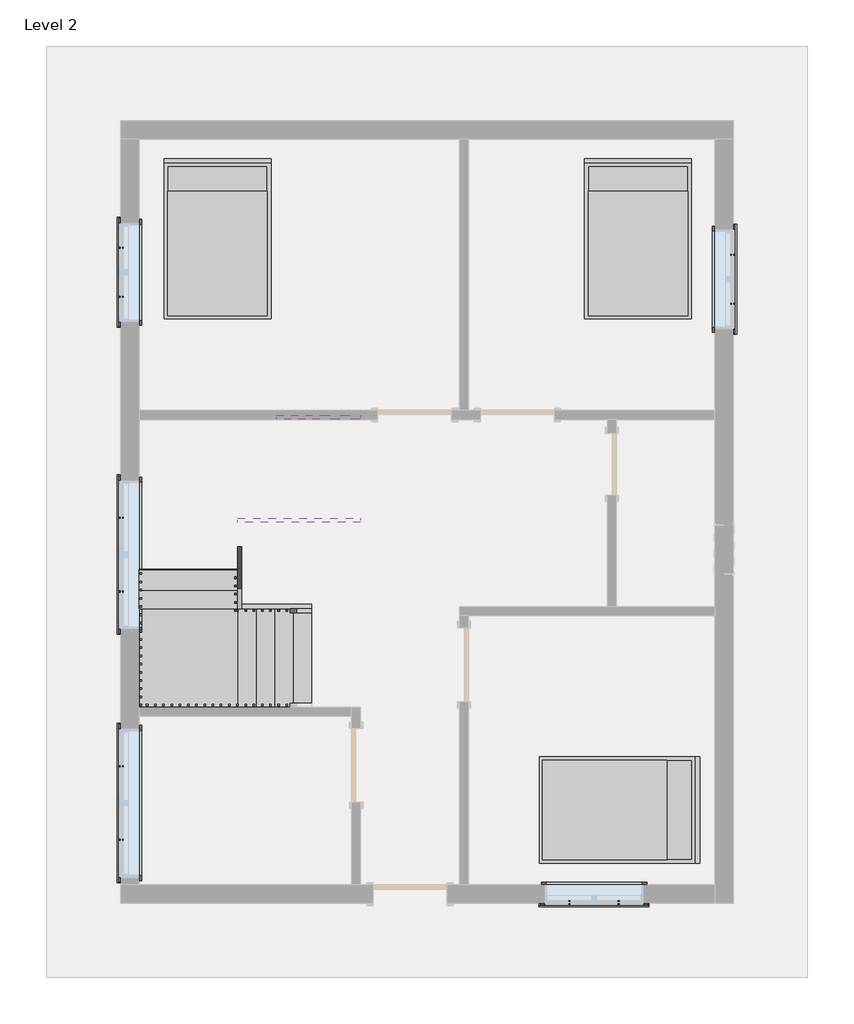
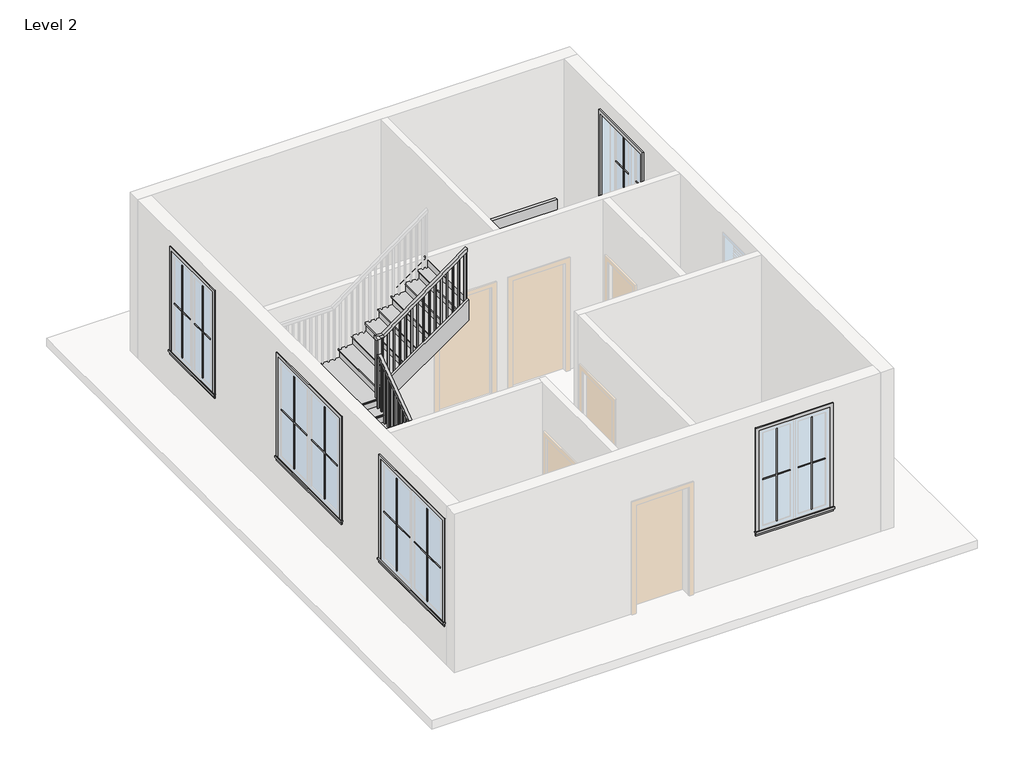
# One storey, part 3 of 3: 20 proxies, 5 members, 3 furniture elements, 1 railing, 1 stair flight.
"""IFC4 building model written with IfcOpenShell, lengths in millimetres."""

from ifc_helpers import new_model, si_unit, frame, origin, place, context, project, spatial, polyline, outline, extrude, faceted_brep, transform, mapped, element, save
from components import muntin_pattern_2x2_muntin_pattern_2x2_0a037076, muntin_pattern_2x2_muntin_pattern_2x2_e6f69628, muntin_pattern_2x2_muntin_pattern_2x2_2b4d9f72, muntin_pattern_2x2_muntin_pattern_2x2_ef995ed3, trim_window_exterior_flat_with_sill_b601e94a, trim_window_exterior_flat_with_sill_b7e4d11c, trim_window_interior_flat_picture_frame_bfefb25c, trim_window_interior_flat_picture_frame_936b8d2a, bed_17739_bed_17739_15c61121, stair_flight_7559bbc3

model = new_model("IFC4")

# Units and contexts
model_context = context("Model", 3, world=origin())
ifc_project = project(units=[si_unit("LENGTHUNIT", "METRE", prefix="MILLI")], contexts=[model_context])

# Site, building, storey
site = spatial("IfcSite", under=ifc_project)
building = spatial("IfcBuilding", under=site)
storey = spatial("IfcBuildingStorey", under=building, Name="Level 2", Elevation=3048.0)

# Proxies
placement = place(None, origin())
muntin_pattern_2x2_muntin_pattern_2x2_shape = muntin_pattern_2x2_muntin_pattern_2x2_0a037076(model_context)
element("IfcBuildingElementProxy", 1, Name="Muntin Pattern_2x2 : Muntin Pattern_2x2", ObjectType="Muntin Pattern_2x2 : Muntin Pattern_2x2", at=placement, inside=storey, context=model_context, shape_type="MappedRepresentation", body=[
    mapped(muntin_pattern_2x2_muntin_pattern_2x2_shape, transform((-5035.7855391, -4380.9248761, 4032.25), x_axis=(0.0, 1.0, 0.0), y_axis=(-1.0, 0.0, 0.0), z_axis=(0.0, 0.0, 1.0))),
])
element("IfcBuildingElementProxy", 2, Name="Muntin Pattern_2x2 : Muntin Pattern_2x2", ObjectType="Muntin Pattern_2x2 : Muntin Pattern_2x2", at=placement, inside=storey, context=model_context, shape_type="MappedRepresentation", body=[
    mapped(muntin_pattern_2x2_muntin_pattern_2x2_shape, transform((-5035.7855391, -1310.6998761, 4032.25), x_axis=(0.0, 1.0, 0.0), y_axis=(-1.0, 0.0, 0.0), z_axis=(0.0, 0.0, 1.0))),
])
muntin_pattern_2x2_muntin_pattern_2x2_2_shape = muntin_pattern_2x2_muntin_pattern_2x2_e6f69628(model_context)
element("IfcBuildingElementProxy", 3, Name="Muntin Pattern_2x2 : Muntin Pattern_2x2", ObjectType="Muntin Pattern_2x2 : Muntin Pattern_2x2", at=placement, inside=storey, context=model_context, shape_type="MappedRepresentation", body=[
    mapped(muntin_pattern_2x2_muntin_pattern_2x2_2_shape, transform((-5035.7855391, -3469.6998761, 4032.25), x_axis=(0.0, -1.0, 0.0), y_axis=(1.0, 0.0, 0.0), z_axis=(0.0, 0.0, 1.0))),
])
element("IfcBuildingElementProxy", 4, Name="Muntin Pattern_2x2 : Muntin Pattern_2x2", ObjectType="Muntin Pattern_2x2 : Muntin Pattern_2x2", at=placement, inside=storey, context=model_context, shape_type="MappedRepresentation", body=[
    mapped(muntin_pattern_2x2_muntin_pattern_2x2_2_shape, transform((-5035.7855391, -399.4748761, 4032.25), x_axis=(0.0, -1.0, 0.0), y_axis=(1.0, 0.0, 0.0), z_axis=(0.0, 0.0, 1.0))),
])
muntin_pattern_2x2_muntin_pattern_2x2_3_shape = muntin_pattern_2x2_muntin_pattern_2x2_2b4d9f72(model_context)
element("IfcBuildingElementProxy", 5, Name="Muntin Pattern_2x2 : Muntin Pattern_2x2", ObjectType="Muntin Pattern_2x2 : Muntin Pattern_2x2", at=placement, inside=storey, context=model_context, shape_type="MappedRepresentation", body=[
    mapped(muntin_pattern_2x2_muntin_pattern_2x2_3_shape, transform((1115.7769609, -5157.2123761, 4032.25), x_axis=(-1.0, 0.0, 0.0), y_axis=(0.0, -1.0, 0.0), z_axis=(0.0, 0.0, 1.0))),
])
element("IfcBuildingElementProxy", 6, Name="Muntin Pattern_2x2 : Muntin Pattern_2x2", ObjectType="Muntin Pattern_2x2 : Muntin Pattern_2x2", at=placement, inside=storey, context=model_context, shape_type="MappedRepresentation", body=[
    mapped(muntin_pattern_2x2_muntin_pattern_2x2_3_shape, transform((2527.0644609, 2851.7251239, 4032.25), x_axis=(0.0, -1.0, 0.0), y_axis=(1.0, 0.0, 0.0), z_axis=(0.0, 0.0, 1.0))),
])
element("IfcBuildingElementProxy", 7, Name="Muntin Pattern_2x2 : Muntin Pattern_2x2", ObjectType="Muntin Pattern_2x2 : Muntin Pattern_2x2", at=placement, inside=storey, context=model_context, shape_type="MappedRepresentation", body=[
    mapped(muntin_pattern_2x2_muntin_pattern_2x2_3_shape, transform((-5035.7855391, 2331.0251239, 4032.25), x_axis=(0.0, 1.0, 0.0), y_axis=(-1.0, 0.0, 0.0), z_axis=(0.0, 0.0, 1.0))),
])
muntin_pattern_2x2_muntin_pattern_2x2_4_shape = muntin_pattern_2x2_muntin_pattern_2x2_ef995ed3(model_context)
element("IfcBuildingElementProxy", 8, Name="Muntin Pattern_2x2 : Muntin Pattern_2x2", ObjectType="Muntin Pattern_2x2 : Muntin Pattern_2x2", at=placement, inside=storey, context=model_context, shape_type="MappedRepresentation", body=[
    mapped(muntin_pattern_2x2_muntin_pattern_2x2_4_shape, transform((509.3519609, -5157.2123761, 4032.25), x_axis=(1.0, 0.0, 0.0), y_axis=(0.0, 1.0, 0.0), z_axis=(0.0, 0.0, 1.0))),
])
element("IfcBuildingElementProxy", 9, Name="Muntin Pattern_2x2 : Muntin Pattern_2x2", ObjectType="Muntin Pattern_2x2 : Muntin Pattern_2x2", at=placement, inside=storey, context=model_context, shape_type="MappedRepresentation", body=[
    mapped(muntin_pattern_2x2_muntin_pattern_2x2_4_shape, transform((2527.0644609, 2245.3001239, 4032.25), x_axis=(0.0, 1.0, 0.0), y_axis=(-1.0, 0.0, 0.0), z_axis=(0.0, 0.0, 1.0))),
])
element("IfcBuildingElementProxy", 10, Name="Muntin Pattern_2x2 : Muntin Pattern_2x2", ObjectType="Muntin Pattern_2x2 : Muntin Pattern_2x2", at=placement, inside=storey, context=model_context, shape_type="MappedRepresentation", body=[
    mapped(muntin_pattern_2x2_muntin_pattern_2x2_4_shape, transform((-5035.7855391, 2937.4501239, 4032.25), x_axis=(0.0, -1.0, 0.0), y_axis=(1.0, 0.0, 0.0), z_axis=(0.0, 0.0, 1.0))),
])
trim_window_exterior_flat_with_sill_shape = trim_window_exterior_flat_with_sill_b601e94a(model_context)
element("IfcBuildingElementProxy", 11, Name="Trim-Window-Exterior-Flat : with Sill", ObjectType="Trim-Window-Exterior-Flat : with Sill", at=placement, inside=storey, context=model_context, shape_type="MappedRepresentation", body=[
    mapped(trim_window_exterior_flat_with_sill_shape, transform((-5045.3105391, -3925.3123761, 5791.2), x_axis=(0.0, -1.0, 0.0), y_axis=(0.0, 0.0, 1.0), z_axis=(-1.0, 0.0, 0.0))),
])
element("IfcBuildingElementProxy", 12, Name="Trim-Window-Exterior-Flat : with Sill", ObjectType="Trim-Window-Exterior-Flat : with Sill", at=placement, inside=storey, context=model_context, shape_type="MappedRepresentation", body=[
    mapped(trim_window_exterior_flat_with_sill_shape, transform((-5045.3105391, -855.0873761, 5791.2), x_axis=(0.0, -1.0, 0.0), y_axis=(0.0, 0.0, 1.0), z_axis=(-1.0, 0.0, 0.0))),
])
trim_window_exterior_flat_with_sill_2_shape = trim_window_exterior_flat_with_sill_b7e4d11c(model_context)
element("IfcBuildingElementProxy", 13, Name="Trim-Window-Exterior-Flat : with Sill", ObjectType="Trim-Window-Exterior-Flat : with Sill", at=placement, inside=storey, context=model_context, shape_type="MappedRepresentation", body=[
    mapped(trim_window_exterior_flat_with_sill_2_shape, transform((812.5644609, -5166.7373761, 5791.2), x_axis=(1.0, 0.0, 0.0), y_axis=(0.0, 0.0, 1.0), z_axis=(0.0, -1.0, 0.0))),
])
element("IfcBuildingElementProxy", 14, Name="Trim-Window-Exterior-Flat : with Sill", ObjectType="Trim-Window-Exterior-Flat : with Sill", at=placement, inside=storey, context=model_context, shape_type="MappedRepresentation", body=[
    mapped(trim_window_exterior_flat_with_sill_2_shape, transform((2536.5894609, 2548.5126239, 5791.2), x_axis=(0.0, 1.0, 0.0), y_axis=(0.0, 0.0, 1.0), z_axis=(1.0, 0.0, 0.0))),
])
element("IfcBuildingElementProxy", 15, Name="Trim-Window-Exterior-Flat : with Sill", ObjectType="Trim-Window-Exterior-Flat : with Sill", at=placement, inside=storey, context=model_context, shape_type="MappedRepresentation", body=[
    mapped(trim_window_exterior_flat_with_sill_2_shape, transform((-5045.3105391, 2634.2376239, 5791.2), x_axis=(0.0, -1.0, 0.0), y_axis=(0.0, 0.0, 1.0), z_axis=(-1.0, 0.0, 0.0))),
])
trim_window_interior_flat_picture_frame_shape = trim_window_interior_flat_picture_frame_bfefb25c(model_context)
element("IfcBuildingElementProxy", 16, Name="Trim-Window-Interior-Flat : Picture Frame", ObjectType="Trim-Window-Interior-Flat : Picture Frame", at=placement, inside=storey, context=model_context, shape_type="MappedRepresentation", body=[
    mapped(trim_window_interior_flat_picture_frame_shape, transform((-4816.7105391, -3925.3123761, 5791.2), x_axis=(0.0, 1.0, 0.0), y_axis=(0.0, 0.0, 1.0), z_axis=(1.0, 0.0, 0.0))),
])
element("IfcBuildingElementProxy", 17, Name="Trim-Window-Interior-Flat : Picture Frame", ObjectType="Trim-Window-Interior-Flat : Picture Frame", at=placement, inside=storey, context=model_context, shape_type="MappedRepresentation", body=[
    mapped(trim_window_interior_flat_picture_frame_shape, transform((-4816.7105391, -855.0873761, 5791.2), x_axis=(0.0, 1.0, 0.0), y_axis=(0.0, 0.0, 1.0), z_axis=(1.0, 0.0, 0.0))),
])
trim_window_interior_flat_picture_frame_2_shape = trim_window_interior_flat_picture_frame_936b8d2a(model_context)
element("IfcBuildingElementProxy", 18, Name="Trim-Window-Interior-Flat : Picture Frame", ObjectType="Trim-Window-Interior-Flat : Picture Frame", at=placement, inside=storey, context=model_context, shape_type="MappedRepresentation", body=[
    mapped(trim_window_interior_flat_picture_frame_2_shape, transform((812.5644609, -4938.1373761, 5791.2), x_axis=(-1.0, 0.0, 0.0), y_axis=(0.0, 0.0, 1.0), z_axis=(0.0, 1.0, 0.0))),
])
element("IfcBuildingElementProxy", 19, Name="Trim-Window-Interior-Flat : Picture Frame", ObjectType="Trim-Window-Interior-Flat : Picture Frame", at=placement, inside=storey, context=model_context, shape_type="MappedRepresentation", body=[
    mapped(trim_window_interior_flat_picture_frame_2_shape, transform((2307.9894609, 2548.5126239, 5791.2), x_axis=(0.0, -1.0, 0.0), y_axis=(0.0, 0.0, 1.0), z_axis=(-1.0, 0.0, 0.0))),
])
element("IfcBuildingElementProxy", 20, Name="Trim-Window-Interior-Flat : Picture Frame", ObjectType="Trim-Window-Interior-Flat : Picture Frame", at=placement, inside=storey, context=model_context, shape_type="MappedRepresentation", body=[
    mapped(trim_window_interior_flat_picture_frame_2_shape, transform((-4816.7105391, 2634.2376239, 5791.2), x_axis=(0.0, 1.0, 0.0), y_axis=(0.0, 0.0, 1.0), z_axis=(1.0, 0.0, 0.0))),
])

# Furniture
bed_17739_bed_17739_shape = bed_17739_bed_17739_15c61121(model_context)
element("IfcFurniture", 21, ObjectType="Bed_17739 : Bed_17739", at=placement, inside=storey, context=model_context, shape_type="MappedRepresentation", body=[
    mapped(bed_17739_bed_17739_shape, transform((-3845.1605391, 3024.7626239, 3048.0), x_axis=(1.0, 0.0, 0.0), y_axis=(0.0, 1.0, 0.0), z_axis=(0.0, 0.0, 1.0))),
])
element("IfcFurniture", 22, ObjectType="Bed_17739 : Bed_17739", at=placement, inside=storey, context=model_context, shape_type="MappedRepresentation", body=[
    mapped(bed_17739_bed_17739_shape, transform((1355.4894609, 3024.7626239, 3048.0), x_axis=(1.0, 0.0, 0.0), y_axis=(0.0, 1.0, 0.0), z_axis=(0.0, 0.0, 1.0))),
])
element("IfcFurniture", 23, ObjectType="Bed_17739 : Bed_17739", at=placement, inside=storey, context=model_context, shape_type="MappedRepresentation", body=[
    mapped(bed_17739_bed_17739_shape, transform((1101.4894609, -4011.0373761, 3048.0), x_axis=(0.0, -1.0, 0.0), y_axis=(1.0, 0.0, 0.0), z_axis=(0.0, 0.0, 1.0))),
])

# Members
element("IfcMember", 24, ObjectType="Stringer - 2\" Width", at=placement, inside=storey, context=model_context, shape_type="SweptSolid", body=[
    extrude(outline(polyline([(3048.0, -2683.1105391), (3198.5087903, -2683.1105391), (3198.5087903, -3112.2707489), (3048.0, -2897.7957228), (3048.0, -2683.1105391)])), frame((0.0, -2791.8373761, 0.0), z_axis=(0.0, 1.0, 0.0), x_axis=(0.0, 0.0, 1.0)), (0.0, 0.0, 1.0), 50.8),
])
element("IfcMember", 25, ObjectType="Stringer - 2\" Width", at=placement, inside=storey, context=model_context, shape_type="SweptSolid", body=[
    extrude(outline(polyline([(5375.4856495, -2580.7583047), (5731.4489938, -2073.5105391), (6103.8117181, -2073.5105391), (5375.4856495, -3111.3751869), (5375.4856495, -2580.7583047)])), frame((0.0, 814.9626239, 0.0), z_axis=(0.0, 1.0, 0.0), x_axis=(0.0, 0.0, 1.0)), (0.0, 0.0, 1.0), 50.8),
])
element("IfcMember", 26, ObjectType="Stringer - 2\" Width", at=placement, inside=storey, context=model_context, shape_type="SweptSolid", body=[
    extrude(outline(polyline([(3048.0, -2683.1105391), (3269.706455, -2683.1105391), (3875.7415427, -3546.7105391), (3503.3788184, -3546.7105391), (3048.0, -2897.7957228), (3048.0, -2683.1105391)])), frame((0.0, -1521.8373761, 0.0), z_axis=(0.0, 1.0, 0.0), x_axis=(0.0, 0.0, 1.0)), (0.0, 0.0, 1.0), 50.8),
])
element("IfcMember", 27, ObjectType="Stringer - 2\" Width", at=placement, inside=storey, context=model_context, shape_type="SweptSolid", body=[
    extrude(outline(polyline([(-1521.8373761, 3698.3564629), (-1521.8373761, 4073.5327137), (-455.0373761, 4839.1786467), (-455.0373761, 4464.0023959), (-1521.8373761, 3698.3564629)])), frame((-3597.5105391, 0.0, 0.0), z_axis=(1.0, 0.0, 0.0), x_axis=(0.0, 1.0, 0.0)), (0.0, 0.0, 1.0), 50.8),
])
element("IfcMember", 28, ObjectType="Stringer - 2\" Width", at=placement, inside=storey, context=model_context, shape_type="SweptSolid", body=[
    extrude(outline(polyline([(5034.3380339, -3597.5105391), (4661.9753096, -3597.5105391), (5731.4489938, -2073.5105391), (6103.8117181, -2073.5105391), (5034.3380339, -3597.5105391)])), frame((0.0, -455.0373761, 0.0), z_axis=(0.0, 1.0, 0.0), x_axis=(0.0, 0.0, 1.0)), (0.0, 0.0, 1.0), 50.8),
])

# Railing
element("IfcRailing", 29, ObjectType="Handrail - Rectangular", at=placement, inside=storey, context=model_context, shape_type="SolidModel", body=[
    faceted_brep([(-2683.1105391, -1572.6373761, 4122.8210526), (-2683.1105391, -1572.6373761, 4060.7605986), (-2683.1105391, -1521.8373761, 4060.7605986), (-2683.1105391, -1521.8373761, 4122.8210526), (-3521.3105391, -1572.6373761, 4711.0315789), (-3572.1105391, -1572.6373761, 4684.6202477), (-3572.1105391, -1521.8373761, 4684.6202477), (-3521.3105391, -1521.8373761, 4711.0315789), (-3521.3105391, -1572.6373761, 4979.615311), (-3572.1105391, -1572.6373761, 4928.815311), (-3572.1105391, -1521.8373761, 4928.815311), (-3521.3105391, -1521.8373761, 4979.615311), (-3648.3105391, -1572.6373761, 4979.615311), (-3648.3105391, -1572.6373761, 4928.815311), (-3597.5105391, -1521.8373761, 4928.815311), (-3597.5105391, -1521.8373761, 4979.615311), (-3648.3105391, -1445.6373761, 4979.615311), (-3648.3105391, -1429.2944467, 4928.815311), (-3597.5105391, -1429.2944467, 4928.815311), (-3597.5105391, -1445.6373761, 4979.615311), (-3648.3105391, -480.4373761, 5672.3425837), (-3648.3105391, -429.6373761, 5646.2725387), (-3597.5105391, -429.6373761, 5646.2725387), (-3597.5105391, -480.4373761, 5672.3425837), (-3648.3105391, -480.4373761, 5943.6), (-3648.3105391, -429.6373761, 5892.8), (-3597.5105391, -429.6373761, 5892.8), (-3597.5105391, -480.4373761, 5943.6), (-3648.3105391, -353.4373761, 5943.6), (-3648.3105391, -353.4373761, 5892.8), (-3597.5105391, -404.2373761, 5892.8), (-3597.5105391, -404.2373761, 5943.6), (-3521.3105391, -353.4373761, 5943.6), (-3504.6160355, -353.4373761, 5892.8), (-3504.6160355, -404.2373761, 5892.8), (-3521.3105391, -404.2373761, 5943.6), (-2073.5105391, -353.4373761, 7010.4), (-2073.5105391, -404.2373761, 7010.4), (-2073.5105391, -404.2373761, 6947.2987868), (-2073.5105391, -353.4373761, 6947.2987868)], [[[0, 1, 2, 3]], [[1, 0, 4, 5]], [[2, 1, 5, 6]], [[3, 2, 6, 7]], [[0, 3, 7, 4]], [[5, 4, 8, 9]], [[6, 5, 9, 10]], [[7, 6, 10, 11]], [[4, 7, 11, 8]], [[9, 8, 12, 13]], [[10, 9, 13, 14]], [[11, 10, 14, 15]], [[8, 11, 15, 12]], [[13, 12, 16, 17]], [[14, 13, 17, 18]], [[15, 14, 18, 19]], [[12, 15, 19, 16]], [[17, 16, 20, 21]], [[18, 17, 21, 22]], [[19, 18, 22, 23]], [[16, 19, 23, 20]], [[21, 20, 24, 25]], [[22, 21, 25, 26]], [[23, 22, 26, 27]], [[20, 23, 27, 24]], [[25, 24, 28, 29]], [[26, 25, 29, 30]], [[27, 26, 30, 31]], [[24, 27, 31, 28]], [[29, 28, 32, 33]], [[30, 29, 33, 34]], [[31, 30, 34, 35]], [[28, 31, 35, 32]], [[36, 37, 38, 39]], [[33, 32, 36, 39]], [[34, 33, 39, 38]], [[35, 34, 38, 37]], [[32, 35, 37, 36]]]),
    extrude(outline(polyline([(6935.6014184, -2089.3855391), (6921.5645763, -2108.4355391), (5935.5789474, -2108.4355391), (5935.5789474, -2089.3855391), (6935.6014184, -2089.3855391)])), frame((0.0, -388.3623761, 0.0), z_axis=(0.0, 1.0, 0.0), x_axis=(0.0, 0.0, 1.0)), (0.0, 0.0, 1.0), 19.05),
    extrude(outline(polyline([(6860.7382605, -2190.9855391), (6846.7014184, -2210.0355391), (5935.5789474, -2210.0355391), (5935.5789474, -2190.9855391), (6860.7382605, -2190.9855391)])), frame((0.0, -388.3623761, 0.0), z_axis=(0.0, 1.0, 0.0), x_axis=(0.0, 0.0, 1.0)), (0.0, 0.0, 1.0), 19.05),
    extrude(outline(polyline([(6785.8751026, -2292.5855391), (6771.8382605, -2311.6355391), (5775.1578947, -2311.6355391), (5775.1578947, -2292.5855391), (6785.8751026, -2292.5855391)])), frame((0.0, -388.3623761, 0.0), z_axis=(0.0, 1.0, 0.0), x_axis=(0.0, 0.0, 1.0)), (0.0, 0.0, 1.0), 19.05),
    extrude(outline(polyline([(6711.0119447, -2394.1855391), (6696.9751026, -2413.2355391), (5775.1578947, -2413.2355391), (5775.1578947, -2394.1855391), (6711.0119447, -2394.1855391)])), frame((0.0, -388.3623761, 0.0), z_axis=(0.0, 1.0, 0.0), x_axis=(0.0, 0.0, 1.0)), (0.0, 0.0, 1.0), 19.05),
    extrude(outline(polyline([(6636.1487868, -2495.7855391), (6622.1119447, -2514.8355391), (5614.7368421, -2514.8355391), (5614.7368421, -2495.7855391), (6636.1487868, -2495.7855391)])), frame((0.0, -388.3623761, 0.0), z_axis=(0.0, 1.0, 0.0), x_axis=(0.0, 0.0, 1.0)), (0.0, 0.0, 1.0), 19.05),
    extrude(outline(polyline([(6561.2856289, -2597.3855391), (6547.2487868, -2616.4355391), (5614.7368421, -2616.4355391), (5614.7368421, -2597.3855391), (6561.2856289, -2597.3855391)])), frame((0.0, -388.3623761, 0.0), z_axis=(0.0, 1.0, 0.0), x_axis=(0.0, 0.0, 1.0)), (0.0, 0.0, 1.0), 19.05),
    extrude(outline(polyline([(6486.422471, -2698.9855391), (6472.3856289, -2718.0355391), (5454.3157895, -2718.0355391), (5454.3157895, -2698.9855391), (6486.422471, -2698.9855391)])), frame((0.0, -388.3623761, 0.0), z_axis=(0.0, 1.0, 0.0), x_axis=(0.0, 0.0, 1.0)), (0.0, 0.0, 1.0), 19.05),
    extrude(outline(polyline([(6411.5593132, -2800.5855391), (6397.522471, -2819.6355391), (5454.3157895, -2819.6355391), (5454.3157895, -2800.5855391), (6411.5593132, -2800.5855391)])), frame((0.0, -388.3623761, 0.0), z_axis=(0.0, 1.0, 0.0), x_axis=(0.0, 0.0, 1.0)), (0.0, 0.0, 1.0), 19.05),
    extrude(outline(polyline([(6336.6961553, -2902.1855391), (6322.6593132, -2921.2355391), (5454.3157895, -2921.2355391), (5454.3157895, -2902.1855391), (6336.6961553, -2902.1855391)])), frame((0.0, -388.3623761, 0.0), z_axis=(0.0, 1.0, 0.0), x_axis=(0.0, 0.0, 1.0)), (0.0, 0.0, 1.0), 19.05),
    extrude(outline(polyline([(6261.8329974, -3003.7855391), (6247.7961553, -3022.8355391), (5293.8947368, -3022.8355391), (5293.8947368, -3003.7855391), (6261.8329974, -3003.7855391)])), frame((0.0, -388.3623761, 0.0), z_axis=(0.0, 1.0, 0.0), x_axis=(0.0, 0.0, 1.0)), (0.0, 0.0, 1.0), 19.05),
    extrude(outline(polyline([(6186.9698395, -3105.3855391), (6172.9329974, -3124.4355391), (5293.8947368, -3124.4355391), (5293.8947368, -3105.3855391), (6186.9698395, -3105.3855391)])), frame((0.0, -388.3623761, 0.0), z_axis=(0.0, 1.0, 0.0), x_axis=(0.0, 0.0, 1.0)), (0.0, 0.0, 1.0), 19.05),
    extrude(outline(polyline([(6112.1066816, -3206.9855391), (6098.0698395, -3226.0355391), (5133.4736842, -3226.0355391), (5133.4736842, -3206.9855391), (6112.1066816, -3206.9855391)])), frame((0.0, -388.3623761, 0.0), z_axis=(0.0, 1.0, 0.0), x_axis=(0.0, 0.0, 1.0)), (0.0, 0.0, 1.0), 19.05),
    extrude(outline(polyline([(6037.2435237, -3308.5855391), (6023.2066816, -3327.6355391), (5133.4736842, -3327.6355391), (5133.4736842, -3308.5855391), (6037.2435237, -3308.5855391)])), frame((0.0, -388.3623761, 0.0), z_axis=(0.0, 1.0, 0.0), x_axis=(0.0, 0.0, 1.0)), (0.0, 0.0, 1.0), 19.05),
    extrude(outline(polyline([(5962.3803658, -3410.1855391), (5948.3435237, -3429.2355391), (4973.0526316, -3429.2355391), (4973.0526316, -3410.1855391), (5962.3803658, -3410.1855391)])), frame((0.0, -388.3623761, 0.0), z_axis=(0.0, 1.0, 0.0), x_axis=(0.0, 0.0, 1.0)), (0.0, 0.0, 1.0), 19.05),
    extrude(outline(polyline([(5887.5172079, -3511.7855391), (5873.4803658, -3530.8355391), (4973.0526316, -3530.8355391), (4973.0526316, -3511.7855391), (5887.5172079, -3511.7855391)])), frame((0.0, -388.3623761, 0.0), z_axis=(0.0, 1.0, 0.0), x_axis=(0.0, 0.0, 1.0)), (0.0, 0.0, 1.0), 19.05),
    extrude(outline(polyline([(-3613.3855391, -439.1623761), (-3632.4355391, -439.1623761), (-3632.4355391, -420.1123761), (-3613.3855391, -420.1123761), (-3613.3855391, -439.1623761)])), frame((0.0, 0.0, 4652.2105263), z_axis=(0.0, 0.0, 1.0), x_axis=(1.0, 0.0, 0.0)), (0.0, 0.0, 1.0), 1240.5894737),
    extrude(outline(polyline([(-540.7623761, 5566.5177541), (-521.7123761, 5580.1900029), (-521.7123761, 4652.2105263), (-540.7623761, 4652.2105263), (-540.7623761, 5566.5177541)])), frame((-3632.4355391, 0.0, 0.0), z_axis=(1.0, 0.0, 0.0), x_axis=(0.0, 1.0, 0.0)), (0.0, 0.0, 1.0), 19.05),
    extrude(outline(polyline([(-642.3623761, 5493.5990938), (-623.3123761, 5507.2713426), (-623.3123761, 4491.7894737), (-642.3623761, 4491.7894737), (-642.3623761, 5493.5990938)])), frame((-3632.4355391, 0.0, 0.0), z_axis=(1.0, 0.0, 0.0), x_axis=(0.0, 1.0, 0.0)), (0.0, 0.0, 1.0), 19.05),
    extrude(outline(polyline([(-743.9623761, 5420.6804335), (-724.9123761, 5434.3526823), (-724.9123761, 4491.7894737), (-743.9623761, 4491.7894737), (-743.9623761, 5420.6804335)])), frame((-3632.4355391, 0.0, 0.0), z_axis=(1.0, 0.0, 0.0), x_axis=(0.0, 1.0, 0.0)), (0.0, 0.0, 1.0), 19.05),
    extrude(outline(polyline([(-845.5623761, 5347.7617732), (-826.5123761, 5361.434022), (-826.5123761, 4491.7894737), (-845.5623761, 4491.7894737), (-845.5623761, 5347.7617732)])), frame((-3632.4355391, 0.0, 0.0), z_axis=(1.0, 0.0, 0.0), x_axis=(0.0, 1.0, 0.0)), (0.0, 0.0, 1.0), 19.05),
    extrude(outline(polyline([(-947.1623761, 5274.8431129), (-928.1123761, 5288.5153617), (-928.1123761, 4331.3684211), (-947.1623761, 4331.3684211), (-947.1623761, 5274.8431129)])), frame((-3632.4355391, 0.0, 0.0), z_axis=(1.0, 0.0, 0.0), x_axis=(0.0, 1.0, 0.0)), (0.0, 0.0, 1.0), 19.05),
    extrude(outline(polyline([(-1048.7623761, 5201.9244526), (-1029.7123761, 5215.5967014), (-1029.7123761, 4331.3684211), (-1048.7623761, 4331.3684211), (-1048.7623761, 5201.9244526)])), frame((-3632.4355391, 0.0, 0.0), z_axis=(1.0, 0.0, 0.0), x_axis=(0.0, 1.0, 0.0)), (0.0, 0.0, 1.0), 19.05),
    extrude(outline(polyline([(-1150.3623761, 5129.0057923), (-1131.3123761, 5142.6780411), (-1131.3123761, 4170.9473684), (-1150.3623761, 4170.9473684), (-1150.3623761, 5129.0057923)])), frame((-3632.4355391, 0.0, 0.0), z_axis=(1.0, 0.0, 0.0), x_axis=(0.0, 1.0, 0.0)), (0.0, 0.0, 1.0), 19.05),
    extrude(outline(polyline([(-1251.9623761, 5056.087132), (-1232.9123761, 5069.7593808), (-1232.9123761, 4170.9473684), (-1251.9623761, 4170.9473684), (-1251.9623761, 5056.087132)])), frame((-3632.4355391, 0.0, 0.0), z_axis=(1.0, 0.0, 0.0), x_axis=(0.0, 1.0, 0.0)), (0.0, 0.0, 1.0), 19.05),
    extrude(outline(polyline([(-1353.5623761, 4983.1684718), (-1334.5123761, 4996.8407206), (-1334.5123761, 4010.5263158), (-1353.5623761, 4010.5263158), (-1353.5623761, 4983.1684718)])), frame((-3632.4355391, 0.0, 0.0), z_axis=(1.0, 0.0, 0.0), x_axis=(0.0, 1.0, 0.0)), (0.0, 0.0, 1.0), 19.05),
    extrude(outline(polyline([(-1455.1623761, 4910.2498115), (-1436.1123761, 4923.9220603), (-1436.1123761, 4010.5263158), (-1455.1623761, 4010.5263158), (-1455.1623761, 4910.2498115)])), frame((-3632.4355391, 0.0, 0.0), z_axis=(1.0, 0.0, 0.0), x_axis=(0.0, 1.0, 0.0)), (0.0, 0.0, 1.0), 19.05),
    extrude(outline(polyline([(-3587.9855391, -1537.7123761), (-3587.9855391, -1556.7623761), (-3607.0355391, -1556.7623761), (-3607.0355391, -1537.7123761), (-3587.9855391, -1537.7123761)])), frame((0.0, 0.0, 3850.1052632), z_axis=(0.0, 0.0, 1.0), x_axis=(1.0, 0.0, 0.0)), (0.0, 0.0, 1.0), 1078.7100478),
    extrude(outline(polyline([(4624.462353, -3486.3855391), (4637.830774, -3505.4355391), (3689.6842105, -3505.4355391), (3689.6842105, -3486.3855391), (4624.462353, -3486.3855391)])), frame((0.0, -1556.7623761, 0.0), z_axis=(0.0, 1.0, 0.0), x_axis=(0.0, 0.0, 1.0)), (0.0, 0.0, 1.0), 19.05),
    extrude(outline(polyline([(4553.1641074, -3384.7855391), (4566.5325284, -3403.8355391), (3689.6842105, -3403.8355391), (3689.6842105, -3384.7855391), (4553.1641074, -3384.7855391)])), frame((0.0, -1556.7623761, 0.0), z_axis=(0.0, 1.0, 0.0), x_axis=(0.0, 0.0, 1.0)), (0.0, 0.0, 1.0), 19.05),
    extrude(outline(polyline([(4481.8658617, -3283.1855391), (4495.2342828, -3302.2355391), (3529.2631579, -3302.2355391), (3529.2631579, -3283.1855391), (4481.8658617, -3283.1855391)])), frame((0.0, -1556.7623761, 0.0), z_axis=(0.0, 1.0, 0.0), x_axis=(0.0, 0.0, 1.0)), (0.0, 0.0, 1.0), 19.05),
    extrude(outline(polyline([(4410.5676161, -3181.5855391), (4423.9360372, -3200.6355391), (3529.2631579, -3200.6355391), (3529.2631579, -3181.5855391), (4410.5676161, -3181.5855391)])), frame((0.0, -1556.7623761, 0.0), z_axis=(0.0, 1.0, 0.0), x_axis=(0.0, 0.0, 1.0)), (0.0, 0.0, 1.0), 19.05),
    extrude(outline(polyline([(4339.2693705, -3079.9855391), (4352.6377916, -3099.0355391), (3368.8421053, -3099.0355391), (3368.8421053, -3079.9855391), (4339.2693705, -3079.9855391)])), frame((0.0, -1556.7623761, 0.0), z_axis=(0.0, 1.0, 0.0), x_axis=(0.0, 0.0, 1.0)), (0.0, 0.0, 1.0), 19.05),
    extrude(outline(polyline([(4267.9711249, -2978.3855391), (4281.3395459, -2997.4355391), (3368.8421053, -2997.4355391), (3368.8421053, -2978.3855391), (4267.9711249, -2978.3855391)])), frame((0.0, -1556.7623761, 0.0), z_axis=(0.0, 1.0, 0.0), x_axis=(0.0, 0.0, 1.0)), (0.0, 0.0, 1.0), 19.05),
    extrude(outline(polyline([(4196.6728793, -2876.7855391), (4210.0413003, -2895.8355391), (3208.4210526, -2895.8355391), (3208.4210526, -2876.7855391), (4196.6728793, -2876.7855391)])), frame((0.0, -1556.7623761, 0.0), z_axis=(0.0, 1.0, 0.0), x_axis=(0.0, 0.0, 1.0)), (0.0, 0.0, 1.0), 19.05),
    extrude(outline(polyline([(4125.3746337, -2775.1855391), (4138.7430547, -2794.2355391), (3208.4210526, -2794.2355391), (3208.4210526, -2775.1855391), (4125.3746337, -2775.1855391)])), frame((0.0, -1556.7623761, 0.0), z_axis=(0.0, 1.0, 0.0), x_axis=(0.0, 0.0, 1.0)), (0.0, 0.0, 1.0), 19.05),
    extrude(outline(polyline([(-3613.3855391, -388.3623761), (-3632.4355391, -388.3623761), (-3632.4355391, -369.3123761), (-3613.3855391, -369.3123761), (-3613.3855391, -388.3623761)])), frame((0.0, 0.0, 4812.6315789), z_axis=(0.0, 0.0, 1.0), x_axis=(1.0, 0.0, 0.0)), (0.0, 0.0, 1.0), 1080.1684211),
    extrude(outline(polyline([(-3613.3855391, -1537.7123761), (-3613.3855391, -1556.7623761), (-3632.4355391, -1556.7623761), (-3632.4355391, -1537.7123761), (-3613.3855391, -1537.7123761)])), frame((0.0, 0.0, 3850.1052632), z_axis=(0.0, 0.0, 1.0), x_axis=(1.0, 0.0, 0.0)), (0.0, 0.0, 1.0), 1078.7100478),
    extrude(outline(polyline([(6947.2987868, -2073.5105391), (6933.2619447, -2092.5605391), (5935.5789474, -2092.5605391), (5935.5789474, -2073.5105391), (6947.2987868, -2073.5105391)])), frame((0.0, -388.3623761, 0.0), z_axis=(0.0, 1.0, 0.0), x_axis=(0.0, 0.0, 1.0)), (0.0, 0.0, 1.0), 19.05),
    extrude(outline(polyline([(4060.7605986, -2683.1105391), (4074.1290196, -2702.1605391), (3208.4210526, -2702.1605391), (3208.4210526, -2683.1105391), (4060.7605986, -2683.1105391)])), frame((0.0, -1556.7623761, 0.0), z_axis=(0.0, 1.0, 0.0), x_axis=(0.0, 0.0, 1.0)), (0.0, 0.0, 1.0), 19.05),
])

# Stair flight
stair_flight_shape = stair_flight_7559bbc3(model_context)
element("IfcStairFlight", 30, ObjectType="2\" Tread 1\" Nosing 1/4\" Riser", at=placement, inside=storey, context=model_context, shape_type="MappedRepresentation", body=[
    mapped(stair_flight_shape, transform((0.0, 0.0, 0.0), x_axis=(1.0, 0.0, 0.0), y_axis=(0.0, 1.0, 0.0), z_axis=(0.0, 0.0, 1.0))),
])

save(model, "model.ifc")

# Revit data of these elements
# Type "Muntin Pattern_2x2 : Muntin Pattern_2x2"
#   Width [instance default] = 4' - 0"
#   Thickness = 0' - 0 1/2"
#   Height [instance default] = 4' - 0"
#   Distance = 0' - 0 3/4"
#   Interior Material [instance default] = none
#   Exterior Material [instance default] = none
#   Default Elevation = 0
# Type "Trim-Window-Exterior-Flat : with Sill"
#   Trim Width = 0' - 2 1/4"
#   Trim Thickness_Picture Frame = 0' - 1 1/4"
#   Trim Thickness_with Sill = 0' - 0 3/4"
#   Sill Thickness = 0' - 1 1/4"
#   Opening Width [instance default] = 2' - 0"
#   Opening Height [instance default] = 3' - 0"
#   Default Elevation = 4' - 0"
#   Sill = yes
#   Picture Frame = no
#   Trim Material [instance default] = none
# Type "Trim-Window-Interior-Flat : Picture Frame"
#   Trim Thickness_Picture Frame = 0' - 1 1/4"
#   Trim Width = 0' - 2 1/4"
#   Trim Thickness_with Sill = 0' - 0 3/4"
#   Sill Thickness = 0' - 1 1/4"
#   Opening Width [instance default] = 2' - 0"
#   Opening Height [instance default] = 3' - 0"
#   Default Elevation = 4' - 0"
#   Sill = no
#   Picture Frame = yes
#   Trim Material [instance default] = none
# Type "Bed_17739 : Bed_17739"
#   Default Elevation = 0
# Type "Handrail - Rectangular"
#   Assembly Code = "C2010400"
#   built-in parameter 1008612 = 0.0416667 (stored number, unit not read)
#   built-in parameter 1008611 = 0.0416667 (stored number, unit not read)
#   built-in parameter 1008609 = 0.333333 (stored number, unit not read)
#   built-in parameter 1008604 = 0.166667 (stored number, unit not read)
#   built-in parameter 1008603 = 0.166667 (stored number, unit not read)
#   Railing Height = 3' - 0"
#   built-in parameter 1008630 = 2
#   built-in parameter 1008610 = 2
#   built-in parameter 1008618 = Baluster - Square : 3/4"
# Elements 1, 2, 3, 4 (IfcBuildingElementProxy, "Muntin Pattern_2x2 : Muntin Pattern_2x2")
#   Width = 2' - 6 5/8"
#   Height = 5' - 6 1/2"
#   Interior Material = Wood - Stained
#   Exterior Material = Clad - White
#   Phase Created = New Construction
#   Materials on its faces: "Clad - White", "Wood - Stained"
# Elements 5, 6, 7, 8, 9, 10 (IfcBuildingElementProxy, "Muntin Pattern_2x2 : Muntin Pattern_2x2")
#   Width = 1' - 6 5/8"
#   Height = 5' - 6 1/2"
#   Interior Material = Wood - Stained
#   Exterior Material = Clad - White
#   Phase Created = New Construction
#   Materials on its faces: "Clad - White", "Wood - Stained"
# Elements 11, 12 (IfcBuildingElementProxy, "Trim-Window-Exterior-Flat : with Sill")
#   Opening Width = 6' - 0"
#   Opening Height = 6' - 0"
#   Trim Material = Clad - White
#   Phase Created = New Construction
#   Materials on its faces: "Clad - White"
# Elements 13, 14, 15 (IfcBuildingElementProxy, "Trim-Window-Exterior-Flat : with Sill")
#   Opening Width = 4' - 0"
#   Opening Height = 6' - 0"
#   Trim Material = Clad - White
#   Phase Created = New Construction
#   Materials on its faces: "Clad - White"
# Elements 16, 17 (IfcBuildingElementProxy, "Trim-Window-Interior-Flat : Picture Frame")
#   Opening Width = 6' - 0"
#   Opening Height = 6' - 0"
#   Trim Material = Wood - Stained
#   Phase Created = New Construction
#   Materials on its faces: "Wood - Stained"
# Elements 18, 19, 20 (IfcBuildingElementProxy, "Trim-Window-Interior-Flat : Picture Frame")
#   Opening Width = 4' - 0"
#   Opening Height = 6' - 0"
#   Trim Material = Wood - Stained
#   Phase Created = New Construction
#   Materials on its faces: "Wood - Stained"
# Elements 21, 22, 23 (IfcFurniture, "Bed_17739 : Bed_17739")
#   Phase Created = New Construction
#   Materials on its faces: "legs", "sheets", "bed frame", "Blanket"
# Elements 24, 25, 26, 27, 28 (IfcMember, "Stringer - 2\" Width")
#   Phase Created = New Construction
# Element 29 (IfcRailing, "Handrail - Rectangular")
#   Phase Created = New Construction
# Element 30 (IfcStairFlight, "2\" Tread 1\" Nosing 1/4\" Riser")
#   Phase Created = New Construction
# Materials
#   "Clad - White": class "Wood", colour RGB 242 242 238, transparency 0, Cost = 0
#   "Wood - Stained": class "Wood", colour RGB 224 178 126, transparency 0, Cost = 0
#   "legs": colour RGB 90 73 37, transparency 0, Cost = 0
#   "sheets": colour RGB 200 195 176, transparency 0, Cost = 0
#   "bed frame": colour RGB 90 73 37, transparency 0, Cost = 0
#   "Blanket": class "System", colour RGB 59 0 1, transparency 0, Cost = 0
